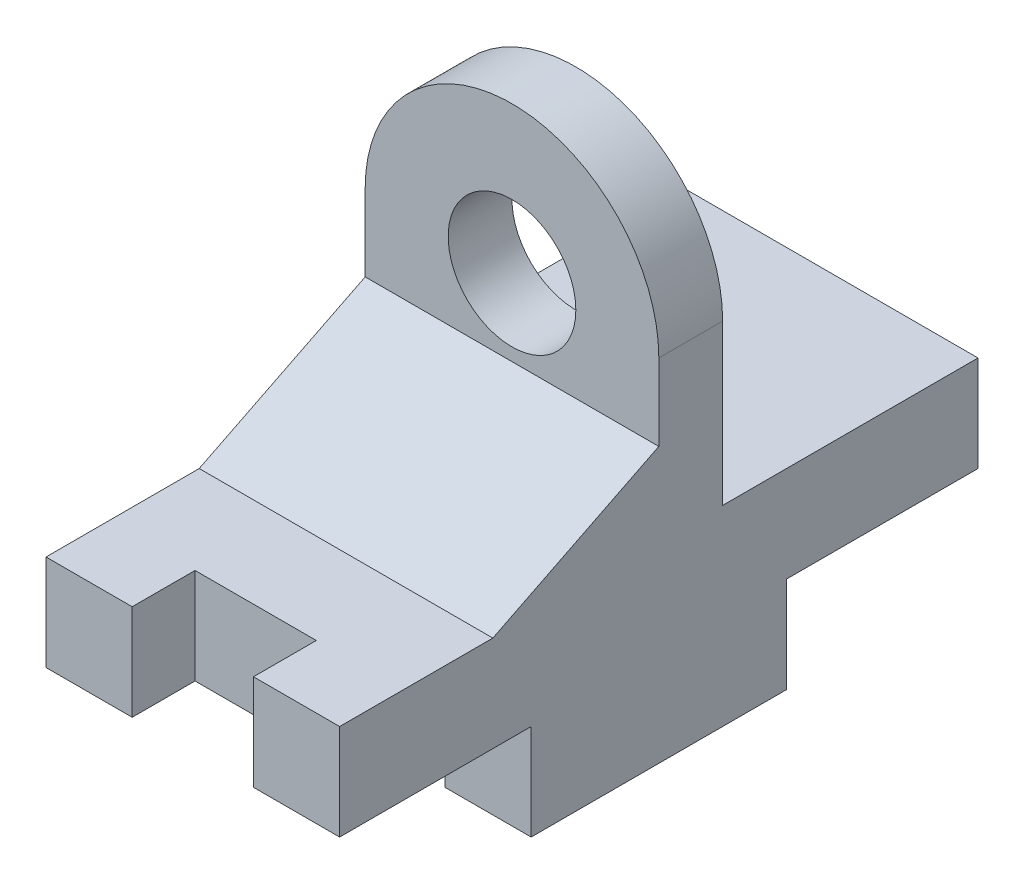
ISO-10303-21;
HEADER;
FILE_DESCRIPTION(('STEP AP214'),'2;1');
FILE_NAME('part.step','',(''),(''),'','','');
FILE_SCHEMA(('AUTOMOTIVE_DESIGN { 1 0 10303 214 1 1 1 1 }'));
ENDSEC;
DATA;
#1=APPLICATION_CONTEXT('core data for automotive mechanical design processes');
#2=APPLICATION_PROTOCOL_DEFINITION('international standard','automotive_design',2000,#1);
#3=PRODUCT_CONTEXT('',#1,'mechanical');
#4=PRODUCT('Part','Part','',(#3));
#5=PRODUCT_RELATED_PRODUCT_CATEGORY('part','',(#4));
#6=PRODUCT_DEFINITION_FORMATION('','',#4);
#7=PRODUCT_DEFINITION_CONTEXT('part definition',#1,'design');
#8=PRODUCT_DEFINITION('design','',#6,#7);
#9=PRODUCT_DEFINITION_SHAPE('','',#8);
#10=(LENGTH_UNIT() NAMED_UNIT(*) SI_UNIT(.MILLI.,.METRE.));
#11=(NAMED_UNIT(*) PLANE_ANGLE_UNIT() SI_UNIT($,.RADIAN.));
#12=(NAMED_UNIT(*) SI_UNIT($,.STERADIAN.) SOLID_ANGLE_UNIT());
#13=UNCERTAINTY_MEASURE_WITH_UNIT(LENGTH_MEASURE(1.E-05),#10,'distance_accuracy_value','');
#14=(GEOMETRIC_REPRESENTATION_CONTEXT(3) GLOBAL_UNCERTAINTY_ASSIGNED_CONTEXT((#13)) GLOBAL_UNIT_ASSIGNED_CONTEXT((#10,
#11,#12)) REPRESENTATION_CONTEXT('',''));
#15=CARTESIAN_POINT('',(0.,0.,0.));
#16=DIRECTION('',(0.,0.,1.));
#17=DIRECTION('',(1.,0.,0.));
#18=AXIS2_PLACEMENT_3D('',#15,#16,#17);
#19=CARTESIAN_POINT('',(0.,15.,0.));
#20=DIRECTION('',(0.,-1.,0.));
#21=DIRECTION('',(0.,0.,-1.));
#22=AXIS2_PLACEMENT_3D('',#19,#20,#21);
#23=PLANE('',#22);
#24=DIRECTION('',(-1.,0.,0.));
#25=VECTOR('',#24,1.);
#26=CARTESIAN_POINT('',(0.,15.,-60.));
#27=LINE('',#26,#25);
#28=CARTESIAN_POINT('',(46.,15.,-60.));
#29=VERTEX_POINT('',#28);
#30=CARTESIAN_POINT('',(0.,15.,-60.));
#31=VERTEX_POINT('',#30);
#32=EDGE_CURVE('E57',#29,#31,#27,.T.);
#33=ORIENTED_EDGE('',*,*,#32,.F.);
#34=DIRECTION('',(0.,0.,-1.));
#35=VECTOR('',#34,1.);
#36=CARTESIAN_POINT('',(46.,15.,0.));
#37=LINE('',#36,#35);
#38=CARTESIAN_POINT('',(46.,15.,-100.));
#39=VERTEX_POINT('',#38);
#40=EDGE_CURVE('E288',#29,#39,#37,.T.);
#41=ORIENTED_EDGE('',*,*,#40,.T.);
#42=DIRECTION('',(-1.,0.,0.));
#43=VECTOR('',#42,1.);
#44=CARTESIAN_POINT('',(0.,15.,-100.));
#45=LINE('',#44,#43);
#46=CARTESIAN_POINT('',(0.,15.,-100.));
#47=VERTEX_POINT('',#46);
#48=EDGE_CURVE('E291',#39,#47,#45,.T.);
#49=ORIENTED_EDGE('',*,*,#48,.T.);
#50=DIRECTION('',(0.,0.,1.));
#51=VECTOR('',#50,1.);
#52=CARTESIAN_POINT('',(0.,15.,0.));
#53=LINE('',#52,#51);
#54=EDGE_CURVE('E280',#47,#31,#53,.T.);
#55=ORIENTED_EDGE('',*,*,#54,.T.);
#56=EDGE_LOOP('',(#33,#41,#49,#55));
#57=FACE_BOUND('',#56,.T.);
#58=ADVANCED_FACE('F41',(#57),#23,.F.);
#59=CARTESIAN_POINT('',(0.,15.,0.));
#60=DIRECTION('',(1.,0.,0.));
#61=DIRECTION('',(0.,0.,-1.));
#62=AXIS2_PLACEMENT_3D('',#59,#60,#61);
#63=PLANE('',#62);
#64=CARTESIAN_POINT('',(0.,15.,-24.));
#65=VERTEX_POINT('',#64);
#66=CARTESIAN_POINT('',(0.,15.,0.));
#67=VERTEX_POINT('',#66);
#68=EDGE_CURVE('E202',#65,#67,#53,.T.);
#69=ORIENTED_EDGE('',*,*,#68,.F.);
#70=DIRECTION('',(0.,-0.447213595499958,0.894427190999916));
#71=VECTOR('',#70,1.);
#72=CARTESIAN_POINT('',(0.,15.,-24.));
#73=LINE('',#72,#71);
#74=CARTESIAN_POINT('',(0.,28.,-50.));
#75=VERTEX_POINT('',#74);
#76=EDGE_CURVE('E190',#75,#65,#73,.T.);
#77=ORIENTED_EDGE('',*,*,#76,.F.);
#78=DIRECTION('',(0.,-1.,0.));
#79=VECTOR('',#78,1.);
#80=CARTESIAN_POINT('',(0.,40.,-50.));
#81=LINE('',#80,#79);
#82=CARTESIAN_POINT('',(0.,40.,-50.));
#83=VERTEX_POINT('',#82);
#84=EDGE_CURVE('E201',#83,#75,#81,.T.);
#85=ORIENTED_EDGE('',*,*,#84,.F.);
#86=DIRECTION('',(0.,0.,1.));
#87=VECTOR('',#86,1.);
#88=CARTESIAN_POINT('',(0.,40.,0.));
#89=LINE('',#88,#87);
#90=CARTESIAN_POINT('',(0.,40.,-60.));
#91=VERTEX_POINT('',#90);
#92=EDGE_CURVE('E208',#91,#83,#89,.T.);
#93=ORIENTED_EDGE('',*,*,#92,.F.);
#94=DIRECTION('',(0.,-1.,0.));
#95=VECTOR('',#94,1.);
#96=CARTESIAN_POINT('',(0.,40.,-60.));
#97=LINE('',#96,#95);
#98=EDGE_CURVE('E209',#91,#31,#97,.T.);
#99=ORIENTED_EDGE('',*,*,#98,.T.);
#100=ORIENTED_EDGE('',*,*,#54,.F.);
#101=DIRECTION('',(0.,-1.,0.));
#102=VECTOR('',#101,1.);
#103=CARTESIAN_POINT('',(0.,15.,-100.));
#104=LINE('',#103,#102);
#105=CARTESIAN_POINT('',(0.,0.,-100.));
#106=VERTEX_POINT('',#105);
#107=EDGE_CURVE('E294',#47,#106,#104,.T.);
#108=ORIENTED_EDGE('',*,*,#107,.T.);
#109=DIRECTION('',(0.,0.,1.));
#110=VECTOR('',#109,1.);
#111=CARTESIAN_POINT('',(0.,0.,0.));
#112=LINE('',#111,#110);
#113=CARTESIAN_POINT('',(0.,0.,-70.));
#114=VERTEX_POINT('',#113);
#115=EDGE_CURVE('E298',#106,#114,#112,.T.);
#116=ORIENTED_EDGE('',*,*,#115,.T.);
#117=DIRECTION('',(0.,1.,0.));
#118=VECTOR('',#117,1.);
#119=CARTESIAN_POINT('',(0.,0.,-70.));
#120=LINE('',#119,#118);
#121=CARTESIAN_POINT('',(0.,-15.,-70.));
#122=VERTEX_POINT('',#121);
#123=EDGE_CURVE('E251',#122,#114,#120,.T.);
#124=ORIENTED_EDGE('',*,*,#123,.F.);
#125=DIRECTION('',(0.,0.,-1.));
#126=VECTOR('',#125,1.);
#127=CARTESIAN_POINT('',(0.,-15.,-70.));
#128=LINE('',#127,#126);
#129=CARTESIAN_POINT('',(0.,-15.,-30.));
#130=VERTEX_POINT('',#129);
#131=EDGE_CURVE('E264',#130,#122,#128,.T.);
#132=ORIENTED_EDGE('',*,*,#131,.F.);
#133=DIRECTION('',(0.,-1.,0.));
#134=VECTOR('',#133,1.);
#135=CARTESIAN_POINT('',(0.,-15.,-30.));
#136=LINE('',#135,#134);
#137=CARTESIAN_POINT('',(0.,0.,-30.));
#138=VERTEX_POINT('',#137);
#139=EDGE_CURVE('E242',#138,#130,#136,.T.);
#140=ORIENTED_EDGE('',*,*,#139,.F.);
#141=CARTESIAN_POINT('',(0.,0.,0.));
#142=VERTEX_POINT('',#141);
#143=EDGE_CURVE('E277',#138,#142,#112,.T.);
#144=ORIENTED_EDGE('',*,*,#143,.T.);
#145=DIRECTION('',(0.,-1.,0.));
#146=VECTOR('',#145,1.);
#147=CARTESIAN_POINT('',(0.,15.,0.));
#148=LINE('',#147,#146);
#149=EDGE_CURVE('E11',#67,#142,#148,.T.);
#150=ORIENTED_EDGE('',*,*,#149,.F.);
#151=EDGE_LOOP('',(#69,#77,#85,#93,#99,#100,#108,#116,#124,#132,#140,#144,#150));
#152=FACE_BOUND('',#151,.T.);
#153=ADVANCED_FACE('F43',(#152),#63,.F.);
#154=CARTESIAN_POINT('',(0.,15.,0.));
#155=DIRECTION('',(0.,0.,-1.));
#156=DIRECTION('',(-1.,0.,0.));
#157=AXIS2_PLACEMENT_3D('',#154,#155,#156);
#158=PLANE('',#157);
#159=DIRECTION('',(1.,0.,0.));
#160=VECTOR('',#159,1.);
#161=CARTESIAN_POINT('',(0.,0.,0.));
#162=LINE('',#161,#160);
#163=CARTESIAN_POINT('',(13.5,0.,0.));
#164=VERTEX_POINT('',#163);
#165=EDGE_CURVE('E299',#142,#164,#162,.T.);
#166=ORIENTED_EDGE('',*,*,#165,.T.);
#167=DIRECTION('',(0.,-1.,0.));
#168=VECTOR('',#167,1.);
#169=CARTESIAN_POINT('',(13.5,15.,0.));
#170=LINE('',#169,#168);
#171=CARTESIAN_POINT('',(13.5,15.,0.));
#172=VERTEX_POINT('',#171);
#173=EDGE_CURVE('E47',#172,#164,#170,.T.);
#174=ORIENTED_EDGE('',*,*,#173,.F.);
#175=DIRECTION('',(1.,0.,0.));
#176=VECTOR('',#175,1.);
#177=CARTESIAN_POINT('',(0.,15.,0.));
#178=LINE('',#177,#176);
#179=EDGE_CURVE('E276',#67,#172,#178,.T.);
#180=ORIENTED_EDGE('',*,*,#179,.F.);
#181=ORIENTED_EDGE('',*,*,#149,.T.);
#182=EDGE_LOOP('',(#166,#174,#180,#181));
#183=FACE_BOUND('',#182,.T.);
#184=ADVANCED_FACE('F360',(#183),#158,.F.);
#185=CARTESIAN_POINT('',(13.5,15.,0.));
#186=DIRECTION('',(-1.,0.,0.));
#187=DIRECTION('',(0.,0.,1.));
#188=AXIS2_PLACEMENT_3D('',#185,#186,#187);
#189=PLANE('',#188);
#190=DIRECTION('',(0.,0.,-1.));
#191=VECTOR('',#190,1.);
#192=CARTESIAN_POINT('',(13.5,0.,0.));
#193=LINE('',#192,#191);
#194=CARTESIAN_POINT('',(13.5,0.,-9.84759162992863));
#195=VERTEX_POINT('',#194);
#196=EDGE_CURVE('E301',#164,#195,#193,.T.);
#197=ORIENTED_EDGE('',*,*,#196,.T.);
#198=DIRECTION('',(0.,-1.,0.));
#199=VECTOR('',#198,1.);
#200=CARTESIAN_POINT('',(13.5,15.,-9.84759162992863));
#201=LINE('',#200,#199);
#202=CARTESIAN_POINT('',(13.5,15.,-9.84759162992863));
#203=VERTEX_POINT('',#202);
#204=EDGE_CURVE('E326',#203,#195,#201,.T.);
#205=ORIENTED_EDGE('',*,*,#204,.F.);
#206=DIRECTION('',(0.,0.,-1.));
#207=VECTOR('',#206,1.);
#208=CARTESIAN_POINT('',(13.5,15.,0.));
#209=LINE('',#208,#207);
#210=EDGE_CURVE('E282',#172,#203,#209,.T.);
#211=ORIENTED_EDGE('',*,*,#210,.F.);
#212=ORIENTED_EDGE('',*,*,#173,.T.);
#213=EDGE_LOOP('',(#197,#205,#211,#212));
#214=FACE_BOUND('',#213,.T.);
#215=ADVANCED_FACE('F337',(#214),#189,.F.);
#216=CARTESIAN_POINT('',(13.5,15.,-9.84759162992863));
#217=DIRECTION('',(0.,0.,-1.));
#218=DIRECTION('',(-1.,0.,0.));
#219=AXIS2_PLACEMENT_3D('',#216,#217,#218);
#220=PLANE('',#219);
#221=DIRECTION('',(1.,0.,0.));
#222=VECTOR('',#221,1.);
#223=CARTESIAN_POINT('',(13.5,0.,-9.84759162992863));
#224=LINE('',#223,#222);
#225=CARTESIAN_POINT('',(32.5,0.,-9.84759162992863));
#226=VERTEX_POINT('',#225);
#227=EDGE_CURVE('E303',#195,#226,#224,.T.);
#228=ORIENTED_EDGE('',*,*,#227,.T.);
#229=DIRECTION('',(0.,-1.,0.));
#230=VECTOR('',#229,1.);
#231=CARTESIAN_POINT('',(32.5,15.,-9.84759162992863));
#232=LINE('',#231,#230);
#233=CARTESIAN_POINT('',(32.5,15.,-9.84759162992863));
#234=VERTEX_POINT('',#233);
#235=EDGE_CURVE('E327',#234,#226,#232,.T.);
#236=ORIENTED_EDGE('',*,*,#235,.F.);
#237=DIRECTION('',(1.,0.,0.));
#238=VECTOR('',#237,1.);
#239=CARTESIAN_POINT('',(13.5,15.,-9.84759162992863));
#240=LINE('',#239,#238);
#241=EDGE_CURVE('E284',#203,#234,#240,.T.);
#242=ORIENTED_EDGE('',*,*,#241,.F.);
#243=ORIENTED_EDGE('',*,*,#204,.T.);
#244=EDGE_LOOP('',(#228,#236,#242,#243));
#245=FACE_BOUND('',#244,.T.);
#246=ADVANCED_FACE('F346',(#245),#220,.F.);
#247=CARTESIAN_POINT('',(32.5,15.,-9.84759162992863));
#248=DIRECTION('',(1.,0.,0.));
#249=DIRECTION('',(0.,0.,-1.));
#250=AXIS2_PLACEMENT_3D('',#247,#248,#249);
#251=PLANE('',#250);
#252=DIRECTION('',(0.,0.,1.));
#253=VECTOR('',#252,1.);
#254=CARTESIAN_POINT('',(32.5,0.,-9.84759162992863));
#255=LINE('',#254,#253);
#256=CARTESIAN_POINT('',(32.5,0.,0.));
#257=VERTEX_POINT('',#256);
#258=EDGE_CURVE('E304',#226,#257,#255,.T.);
#259=ORIENTED_EDGE('',*,*,#258,.T.);
#260=DIRECTION('',(0.,-1.,0.));
#261=VECTOR('',#260,1.);
#262=CARTESIAN_POINT('',(32.5,15.,0.));
#263=LINE('',#262,#261);
#264=CARTESIAN_POINT('',(32.5,15.,0.));
#265=VERTEX_POINT('',#264);
#266=EDGE_CURVE('E324',#265,#257,#263,.T.);
#267=ORIENTED_EDGE('',*,*,#266,.F.);
#268=DIRECTION('',(0.,0.,1.));
#269=VECTOR('',#268,1.);
#270=CARTESIAN_POINT('',(32.5,15.,-9.84759162992863));
#271=LINE('',#270,#269);
#272=EDGE_CURVE('E283',#234,#265,#271,.T.);
#273=ORIENTED_EDGE('',*,*,#272,.F.);
#274=ORIENTED_EDGE('',*,*,#235,.T.);
#275=EDGE_LOOP('',(#259,#267,#273,#274));
#276=FACE_BOUND('',#275,.T.);
#277=ADVANCED_FACE('F352',(#276),#251,.F.);
#278=CARTESIAN_POINT('',(32.5,15.,0.));
#279=DIRECTION('',(0.,0.,-1.));
#280=DIRECTION('',(-1.,0.,0.));
#281=AXIS2_PLACEMENT_3D('',#278,#279,#280);
#282=PLANE('',#281);
#283=DIRECTION('',(1.,0.,0.));
#284=VECTOR('',#283,1.);
#285=CARTESIAN_POINT('',(32.5,0.,0.));
#286=LINE('',#285,#284);
#287=CARTESIAN_POINT('',(46.,0.,0.));
#288=VERTEX_POINT('',#287);
#289=EDGE_CURVE('E310',#257,#288,#286,.T.);
#290=ORIENTED_EDGE('',*,*,#289,.T.);
#291=DIRECTION('',(0.,-1.,0.));
#292=VECTOR('',#291,1.);
#293=CARTESIAN_POINT('',(46.,15.,0.));
#294=LINE('',#293,#292);
#295=CARTESIAN_POINT('',(46.,15.,0.));
#296=VERTEX_POINT('',#295);
#297=EDGE_CURVE('E318',#296,#288,#294,.T.);
#298=ORIENTED_EDGE('',*,*,#297,.F.);
#299=DIRECTION('',(1.,0.,0.));
#300=VECTOR('',#299,1.);
#301=CARTESIAN_POINT('',(32.5,15.,0.));
#302=LINE('',#301,#300);
#303=EDGE_CURVE('E290',#265,#296,#302,.T.);
#304=ORIENTED_EDGE('',*,*,#303,.F.);
#305=ORIENTED_EDGE('',*,*,#266,.T.);
#306=EDGE_LOOP('',(#290,#298,#304,#305));
#307=FACE_BOUND('',#306,.T.);
#308=ADVANCED_FACE('F454',(#307),#282,.F.);
#309=CARTESIAN_POINT('',(46.,15.,0.));
#310=DIRECTION('',(-1.,0.,0.));
#311=DIRECTION('',(0.,0.,1.));
#312=AXIS2_PLACEMENT_3D('',#309,#310,#311);
#313=PLANE('',#312);
#314=DIRECTION('',(0.,0.,-1.));
#315=VECTOR('',#314,1.);
#316=CARTESIAN_POINT('',(46.,0.,0.));
#317=LINE('',#316,#315);
#318=CARTESIAN_POINT('',(46.,0.,-30.));
#319=VERTEX_POINT('',#318);
#320=EDGE_CURVE('E309',#288,#319,#317,.T.);
#321=ORIENTED_EDGE('',*,*,#320,.T.);
#322=DIRECTION('',(0.,-1.,0.));
#323=VECTOR('',#322,1.);
#324=CARTESIAN_POINT('',(46.,-15.,-30.));
#325=LINE('',#324,#323);
#326=CARTESIAN_POINT('',(46.,-15.,-30.));
#327=VERTEX_POINT('',#326);
#328=EDGE_CURVE('E222',#319,#327,#325,.T.);
#329=ORIENTED_EDGE('',*,*,#328,.T.);
#330=DIRECTION('',(0.,0.,-1.));
#331=VECTOR('',#330,1.);
#332=CARTESIAN_POINT('',(46.,-15.,-70.));
#333=LINE('',#332,#331);
#334=CARTESIAN_POINT('',(46.,-15.,-70.));
#335=VERTEX_POINT('',#334);
#336=EDGE_CURVE('E238',#327,#335,#333,.T.);
#337=ORIENTED_EDGE('',*,*,#336,.T.);
#338=DIRECTION('',(0.,1.,0.));
#339=VECTOR('',#338,1.);
#340=CARTESIAN_POINT('',(46.,0.,-70.));
#341=LINE('',#340,#339);
#342=CARTESIAN_POINT('',(46.,0.,-70.));
#343=VERTEX_POINT('',#342);
#344=EDGE_CURVE('E61',#335,#343,#341,.T.);
#345=ORIENTED_EDGE('',*,*,#344,.T.);
#346=CARTESIAN_POINT('',(46.,0.,-100.));
#347=VERTEX_POINT('',#346);
#348=EDGE_CURVE('E307',#343,#347,#317,.T.);
#349=ORIENTED_EDGE('',*,*,#348,.T.);
#350=DIRECTION('',(0.,-1.,0.));
#351=VECTOR('',#350,1.);
#352=CARTESIAN_POINT('',(46.,15.,-100.));
#353=LINE('',#352,#351);
#354=EDGE_CURVE('E320',#39,#347,#353,.T.);
#355=ORIENTED_EDGE('',*,*,#354,.F.);
#356=ORIENTED_EDGE('',*,*,#40,.F.);
#357=DIRECTION('',(0.,-1.,0.));
#358=VECTOR('',#357,1.);
#359=CARTESIAN_POINT('',(46.,40.,-60.));
#360=LINE('',#359,#358);
#361=CARTESIAN_POINT('',(46.,40.,-60.));
#362=VERTEX_POINT('',#361);
#363=EDGE_CURVE('E214',#362,#29,#360,.T.);
#364=ORIENTED_EDGE('',*,*,#363,.F.);
#365=DIRECTION('',(0.,0.,-1.));
#366=VECTOR('',#365,1.);
#367=CARTESIAN_POINT('',(46.,40.,0.));
#368=LINE('',#367,#366);
#369=CARTESIAN_POINT('',(46.,40.,-50.));
#370=VERTEX_POINT('',#369);
#371=EDGE_CURVE('E213',#370,#362,#368,.T.);
#372=ORIENTED_EDGE('',*,*,#371,.F.);
#373=DIRECTION('',(0.,-1.,0.));
#374=VECTOR('',#373,1.);
#375=CARTESIAN_POINT('',(46.,40.,-50.));
#376=LINE('',#375,#374);
#377=CARTESIAN_POINT('',(46.,28.,-50.));
#378=VERTEX_POINT('',#377);
#379=EDGE_CURVE('E221',#370,#378,#376,.T.);
#380=ORIENTED_EDGE('',*,*,#379,.T.);
#381=DIRECTION('',(0.,-0.447213595499958,0.894427190999916));
#382=VECTOR('',#381,1.);
#383=CARTESIAN_POINT('',(46.,15.,-24.));
#384=LINE('',#383,#382);
#385=CARTESIAN_POINT('',(46.,15.,-24.));
#386=VERTEX_POINT('',#385);
#387=EDGE_CURVE('E188',#378,#386,#384,.T.);
#388=ORIENTED_EDGE('',*,*,#387,.T.);
#389=EDGE_CURVE('E289',#296,#386,#37,.T.);
#390=ORIENTED_EDGE('',*,*,#389,.F.);
#391=ORIENTED_EDGE('',*,*,#297,.T.);
#392=EDGE_LOOP('',(#321,#329,#337,#345,#349,#355,#356,#364,#372,#380,#388,#390,#391));
#393=FACE_BOUND('',#392,.T.);
#394=ADVANCED_FACE('F383',(#393),#313,.F.);
#395=CARTESIAN_POINT('',(0.,15.,-100.));
#396=DIRECTION('',(0.,0.,1.));
#397=DIRECTION('',(1.,0.,0.));
#398=AXIS2_PLACEMENT_3D('',#395,#396,#397);
#399=PLANE('',#398);
#400=DIRECTION('',(-1.,0.,0.));
#401=VECTOR('',#400,1.);
#402=CARTESIAN_POINT('',(0.,0.,-100.));
#403=LINE('',#402,#401);
#404=EDGE_CURVE('E312',#347,#106,#403,.T.);
#405=ORIENTED_EDGE('',*,*,#404,.T.);
#406=ORIENTED_EDGE('',*,*,#107,.F.);
#407=ORIENTED_EDGE('',*,*,#48,.F.);
#408=ORIENTED_EDGE('',*,*,#354,.T.);
#409=EDGE_LOOP('',(#405,#406,#407,#408));
#410=FACE_BOUND('',#409,.T.);
#411=ADVANCED_FACE('F382',(#410),#399,.F.);
#412=ORIENTED_EDGE('',*,*,#389,.T.);
#413=DIRECTION('',(1.,0.,0.));
#414=VECTOR('',#413,1.);
#415=CARTESIAN_POINT('',(0.,15.,-24.));
#416=LINE('',#415,#414);
#417=EDGE_CURVE('E193',#65,#386,#416,.T.);
#418=ORIENTED_EDGE('',*,*,#417,.F.);
#419=ORIENTED_EDGE('',*,*,#68,.T.);
#420=ORIENTED_EDGE('',*,*,#179,.T.);
#421=ORIENTED_EDGE('',*,*,#210,.T.);
#422=ORIENTED_EDGE('',*,*,#241,.T.);
#423=ORIENTED_EDGE('',*,*,#272,.T.);
#424=ORIENTED_EDGE('',*,*,#303,.T.);
#425=EDGE_LOOP('',(#412,#418,#419,#420,#421,#422,#423,#424));
#426=FACE_BOUND('',#425,.T.);
#427=ADVANCED_FACE('F357',(#426),#23,.F.);
#428=CARTESIAN_POINT('',(0.,0.,0.));
#429=DIRECTION('',(0.,-1.,0.));
#430=DIRECTION('',(0.,0.,-1.));
#431=AXIS2_PLACEMENT_3D('',#428,#429,#430);
#432=PLANE('',#431);
#433=DIRECTION('',(1.,0.,0.));
#434=VECTOR('',#433,1.);
#435=CARTESIAN_POINT('',(32.5,0.,-30.));
#436=LINE('',#435,#434);
#437=CARTESIAN_POINT('',(32.5,0.,-30.));
#438=VERTEX_POINT('',#437);
#439=EDGE_CURVE('E241',#438,#319,#436,.T.);
#440=ORIENTED_EDGE('',*,*,#439,.T.);
#441=ORIENTED_EDGE('',*,*,#320,.F.);
#442=ORIENTED_EDGE('',*,*,#289,.F.);
#443=ORIENTED_EDGE('',*,*,#258,.F.);
#444=ORIENTED_EDGE('',*,*,#227,.F.);
#445=ORIENTED_EDGE('',*,*,#196,.F.);
#446=ORIENTED_EDGE('',*,*,#165,.F.);
#447=ORIENTED_EDGE('',*,*,#143,.F.);
#448=DIRECTION('',(-1.,0.,0.));
#449=VECTOR('',#448,1.);
#450=CARTESIAN_POINT('',(13.5,0.,-30.));
#451=LINE('',#450,#449);
#452=CARTESIAN_POINT('',(13.5,0.,-30.));
#453=VERTEX_POINT('',#452);
#454=EDGE_CURVE('E258',#453,#138,#451,.T.);
#455=ORIENTED_EDGE('',*,*,#454,.F.);
#456=DIRECTION('',(0.,0.,1.));
#457=VECTOR('',#456,1.);
#458=CARTESIAN_POINT('',(13.5,0.,-30.));
#459=LINE('',#458,#457);
#460=CARTESIAN_POINT('',(13.5,0.,-70.));
#461=VERTEX_POINT('',#460);
#462=EDGE_CURVE('E259',#461,#453,#459,.T.);
#463=ORIENTED_EDGE('',*,*,#462,.F.);
#464=DIRECTION('',(-1.,0.,0.));
#465=VECTOR('',#464,1.);
#466=CARTESIAN_POINT('',(13.5,0.,-70.));
#467=LINE('',#466,#465);
#468=EDGE_CURVE('E270',#461,#114,#467,.T.);
#469=ORIENTED_EDGE('',*,*,#468,.T.);
#470=ORIENTED_EDGE('',*,*,#115,.F.);
#471=ORIENTED_EDGE('',*,*,#404,.F.);
#472=ORIENTED_EDGE('',*,*,#348,.F.);
#473=DIRECTION('',(1.,0.,0.));
#474=VECTOR('',#473,1.);
#475=CARTESIAN_POINT('',(32.5,0.,-70.));
#476=LINE('',#475,#474);
#477=CARTESIAN_POINT('',(32.5,0.,-70.));
#478=VERTEX_POINT('',#477);
#479=EDGE_CURVE('E244',#478,#343,#476,.T.);
#480=ORIENTED_EDGE('',*,*,#479,.F.);
#481=DIRECTION('',(0.,0.,1.));
#482=VECTOR('',#481,1.);
#483=CARTESIAN_POINT('',(32.5,0.,-30.));
#484=LINE('',#483,#482);
#485=EDGE_CURVE('E235',#478,#438,#484,.T.);
#486=ORIENTED_EDGE('',*,*,#485,.T.);
#487=EDGE_LOOP('',(#440,#441,#442,#443,#444,#445,#446,#447,#455,#463,#469,#470,#471,#472,#480,#486));
#488=FACE_BOUND('',#487,.T.);
#489=ADVANCED_FACE('F344',(#488),#432,.T.);
#490=CARTESIAN_POINT('',(13.5,-15.,-30.));
#491=DIRECTION('',(0.,0.,-1.));
#492=DIRECTION('',(0.,1.,0.));
#493=AXIS2_PLACEMENT_3D('',#490,#491,#492);
#494=PLANE('',#493);
#495=ORIENTED_EDGE('',*,*,#139,.T.);
#496=DIRECTION('',(-1.,0.,0.));
#497=VECTOR('',#496,1.);
#498=CARTESIAN_POINT('',(13.5,-15.,-30.));
#499=LINE('',#498,#497);
#500=CARTESIAN_POINT('',(13.5,-15.,-30.));
#501=VERTEX_POINT('',#500);
#502=EDGE_CURVE('E271',#501,#130,#499,.T.);
#503=ORIENTED_EDGE('',*,*,#502,.F.);
#504=DIRECTION('',(0.,-1.,0.));
#505=VECTOR('',#504,1.);
#506=CARTESIAN_POINT('',(13.5,-15.,-30.));
#507=LINE('',#506,#505);
#508=EDGE_CURVE('E249',#453,#501,#507,.T.);
#509=ORIENTED_EDGE('',*,*,#508,.F.);
#510=ORIENTED_EDGE('',*,*,#454,.T.);
#511=EDGE_LOOP('',(#495,#503,#509,#510));
#512=FACE_BOUND('',#511,.T.);
#513=ADVANCED_FACE('F362',(#512),#494,.F.);
#514=CARTESIAN_POINT('',(13.5,-15.,-70.));
#515=DIRECTION('',(0.,1.,0.));
#516=DIRECTION('',(0.,0.,1.));
#517=AXIS2_PLACEMENT_3D('',#514,#515,#516);
#518=PLANE('',#517);
#519=ORIENTED_EDGE('',*,*,#131,.T.);
#520=DIRECTION('',(-1.,0.,0.));
#521=VECTOR('',#520,1.);
#522=CARTESIAN_POINT('',(13.5,-15.,-70.));
#523=LINE('',#522,#521);
#524=CARTESIAN_POINT('',(13.5,-15.,-70.));
#525=VERTEX_POINT('',#524);
#526=EDGE_CURVE('E269',#525,#122,#523,.T.);
#527=ORIENTED_EDGE('',*,*,#526,.F.);
#528=DIRECTION('',(0.,0.,-1.));
#529=VECTOR('',#528,1.);
#530=CARTESIAN_POINT('',(13.5,-15.,-70.));
#531=LINE('',#530,#529);
#532=EDGE_CURVE('E254',#501,#525,#531,.T.);
#533=ORIENTED_EDGE('',*,*,#532,.F.);
#534=ORIENTED_EDGE('',*,*,#502,.T.);
#535=EDGE_LOOP('',(#519,#527,#533,#534));
#536=FACE_BOUND('',#535,.T.);
#537=ADVANCED_FACE('F535',(#536),#518,.F.);
#538=CARTESIAN_POINT('',(13.5,0.,-70.));
#539=DIRECTION('',(0.,0.,1.));
#540=DIRECTION('',(1.,0.,0.));
#541=AXIS2_PLACEMENT_3D('',#538,#539,#540);
#542=PLANE('',#541);
#543=ORIENTED_EDGE('',*,*,#123,.T.);
#544=ORIENTED_EDGE('',*,*,#468,.F.);
#545=DIRECTION('',(0.,1.,0.));
#546=VECTOR('',#545,1.);
#547=CARTESIAN_POINT('',(13.5,0.,-70.));
#548=LINE('',#547,#546);
#549=EDGE_CURVE('E257',#525,#461,#548,.T.);
#550=ORIENTED_EDGE('',*,*,#549,.F.);
#551=ORIENTED_EDGE('',*,*,#526,.T.);
#552=EDGE_LOOP('',(#543,#544,#550,#551));
#553=FACE_BOUND('',#552,.T.);
#554=ADVANCED_FACE('F373',(#553),#542,.F.);
#555=CARTESIAN_POINT('',(13.5,0.,0.));
#556=DIRECTION('',(-1.,0.,0.));
#557=DIRECTION('',(0.,0.,1.));
#558=AXIS2_PLACEMENT_3D('',#555,#556,#557);
#559=PLANE('',#558);
#560=ORIENTED_EDGE('',*,*,#508,.T.);
#561=ORIENTED_EDGE('',*,*,#532,.T.);
#562=ORIENTED_EDGE('',*,*,#549,.T.);
#563=ORIENTED_EDGE('',*,*,#462,.T.);
#564=EDGE_LOOP('',(#560,#561,#562,#563));
#565=FACE_BOUND('',#564,.T.);
#566=ADVANCED_FACE('F368',(#565),#559,.F.);
#567=CARTESIAN_POINT('',(32.5,-15.,-30.));
#568=DIRECTION('',(0.,0.,1.));
#569=DIRECTION('',(0.,-1.,0.));
#570=AXIS2_PLACEMENT_3D('',#567,#568,#569);
#571=PLANE('',#570);
#572=ORIENTED_EDGE('',*,*,#328,.F.);
#573=ORIENTED_EDGE('',*,*,#439,.F.);
#574=DIRECTION('',(0.,-1.,0.));
#575=VECTOR('',#574,1.);
#576=CARTESIAN_POINT('',(32.5,-15.,-30.));
#577=LINE('',#576,#575);
#578=CARTESIAN_POINT('',(32.5,-15.,-30.));
#579=VERTEX_POINT('',#578);
#580=EDGE_CURVE('E223',#438,#579,#577,.T.);
#581=ORIENTED_EDGE('',*,*,#580,.T.);
#582=DIRECTION('',(1.,0.,0.));
#583=VECTOR('',#582,1.);
#584=CARTESIAN_POINT('',(32.5,-15.,-30.));
#585=LINE('',#584,#583);
#586=EDGE_CURVE('E232',#579,#327,#585,.T.);
#587=ORIENTED_EDGE('',*,*,#586,.T.);
#588=EDGE_LOOP('',(#572,#573,#581,#587));
#589=FACE_BOUND('',#588,.T.);
#590=ADVANCED_FACE('F414',(#589),#571,.T.);
#591=CARTESIAN_POINT('',(32.5,0.,-70.));
#592=DIRECTION('',(0.,0.,-1.));
#593=DIRECTION('',(-1.,0.,0.));
#594=AXIS2_PLACEMENT_3D('',#591,#592,#593);
#595=PLANE('',#594);
#596=ORIENTED_EDGE('',*,*,#344,.F.);
#597=DIRECTION('',(1.,0.,0.));
#598=VECTOR('',#597,1.);
#599=CARTESIAN_POINT('',(32.5,-15.,-70.));
#600=LINE('',#599,#598);
#601=CARTESIAN_POINT('',(32.5,-15.,-70.));
#602=VERTEX_POINT('',#601);
#603=EDGE_CURVE('E250',#602,#335,#600,.T.);
#604=ORIENTED_EDGE('',*,*,#603,.F.);
#605=DIRECTION('',(0.,1.,0.));
#606=VECTOR('',#605,1.);
#607=CARTESIAN_POINT('',(32.5,0.,-70.));
#608=LINE('',#607,#606);
#609=EDGE_CURVE('E229',#602,#478,#608,.T.);
#610=ORIENTED_EDGE('',*,*,#609,.T.);
#611=ORIENTED_EDGE('',*,*,#479,.T.);
#612=EDGE_LOOP('',(#596,#604,#610,#611));
#613=FACE_BOUND('',#612,.T.);
#614=ADVANCED_FACE('F422',(#613),#595,.T.);
#615=CARTESIAN_POINT('',(32.5,-15.,-70.));
#616=DIRECTION('',(0.,-1.,0.));
#617=DIRECTION('',(0.,0.,-1.));
#618=AXIS2_PLACEMENT_3D('',#615,#616,#617);
#619=PLANE('',#618);
#620=ORIENTED_EDGE('',*,*,#336,.F.);
#621=ORIENTED_EDGE('',*,*,#586,.F.);
#622=DIRECTION('',(0.,0.,-1.));
#623=VECTOR('',#622,1.);
#624=CARTESIAN_POINT('',(32.5,-15.,-70.));
#625=LINE('',#624,#623);
#626=EDGE_CURVE('E227',#579,#602,#625,.T.);
#627=ORIENTED_EDGE('',*,*,#626,.T.);
#628=ORIENTED_EDGE('',*,*,#603,.T.);
#629=EDGE_LOOP('',(#620,#621,#627,#628));
#630=FACE_BOUND('',#629,.T.);
#631=ADVANCED_FACE('F419',(#630),#619,.T.);
#632=CARTESIAN_POINT('',(32.5,0.,0.));
#633=DIRECTION('',(-1.,0.,0.));
#634=DIRECTION('',(0.,0.,1.));
#635=AXIS2_PLACEMENT_3D('',#632,#633,#634);
#636=PLANE('',#635);
#637=ORIENTED_EDGE('',*,*,#580,.F.);
#638=ORIENTED_EDGE('',*,*,#485,.F.);
#639=ORIENTED_EDGE('',*,*,#609,.F.);
#640=ORIENTED_EDGE('',*,*,#626,.F.);
#641=EDGE_LOOP('',(#637,#638,#639,#640));
#642=FACE_BOUND('',#641,.T.);
#643=ADVANCED_FACE('F416',(#642),#636,.T.);
#644=CARTESIAN_POINT('',(0.,40.,-50.));
#645=DIRECTION('',(0.,0.,1.));
#646=DIRECTION('',(1.,0.,0.));
#647=AXIS2_PLACEMENT_3D('',#644,#645,#646);
#648=PLANE('',#647);
#649=DIRECTION('',(1.,0.,0.));
#650=VECTOR('',#649,1.);
#651=CARTESIAN_POINT('',(0.,28.,-50.));
#652=LINE('',#651,#650);
#653=EDGE_CURVE('E183',#75,#378,#652,.T.);
#654=ORIENTED_EDGE('',*,*,#653,.T.);
#655=ORIENTED_EDGE('',*,*,#379,.F.);
#656=CARTESIAN_POINT('',(23.,40.,-50.));
#657=DIRECTION('',(0.,0.,1.));
#658=DIRECTION('',(1.,0.,0.));
#659=AXIS2_PLACEMENT_3D('',#656,#657,#658);
#660=CIRCLE('',#659,23.);
#661=EDGE_CURVE('E210',#370,#83,#660,.T.);
#662=ORIENTED_EDGE('',*,*,#661,.T.);
#663=ORIENTED_EDGE('',*,*,#84,.T.);
#664=EDGE_LOOP('',(#654,#655,#662,#663));
#665=FACE_BOUND('',#664,.T.);
#666=CARTESIAN_POINT('',(23.,40.,-50.));
#667=DIRECTION('',(0.,0.,1.));
#668=DIRECTION('',(1.,0.,0.));
#669=AXIS2_PLACEMENT_3D('',#666,#667,#668);
#670=CIRCLE('',#669,10.);
#671=CARTESIAN_POINT('',(33.,40.,-50.));
#672=VERTEX_POINT('',#671);
#673=EDGE_CURVE('E399',#672,#672,#670,.T.);
#674=ORIENTED_EDGE('',*,*,#673,.F.);
#675=EDGE_LOOP('',(#674));
#676=FACE_BOUND('',#675,.T.);
#677=ADVANCED_FACE('F204',(#665,#676),#648,.T.);
#678=CARTESIAN_POINT('',(0.,40.,-60.));
#679=DIRECTION('',(0.,0.,1.));
#680=DIRECTION('',(1.,0.,0.));
#681=AXIS2_PLACEMENT_3D('',#678,#679,#680);
#682=PLANE('',#681);
#683=ORIENTED_EDGE('',*,*,#98,.F.);
#684=CARTESIAN_POINT('',(23.,40.,-60.));
#685=DIRECTION('',(0.,0.,1.));
#686=DIRECTION('',(1.,0.,0.));
#687=AXIS2_PLACEMENT_3D('',#684,#685,#686);
#688=CIRCLE('',#687,23.);
#689=EDGE_CURVE('E394',#362,#91,#688,.T.);
#690=ORIENTED_EDGE('',*,*,#689,.F.);
#691=ORIENTED_EDGE('',*,*,#363,.T.);
#692=ORIENTED_EDGE('',*,*,#32,.T.);
#693=EDGE_LOOP('',(#683,#690,#691,#692));
#694=FACE_BOUND('',#693,.T.);
#695=CARTESIAN_POINT('',(23.,40.,-60.));
#696=DIRECTION('',(0.,0.,1.));
#697=DIRECTION('',(1.,0.,0.));
#698=AXIS2_PLACEMENT_3D('',#695,#696,#697);
#699=CIRCLE('',#698,10.);
#700=CARTESIAN_POINT('',(33.,40.,-60.));
#701=VERTEX_POINT('',#700);
#702=EDGE_CURVE('E393',#701,#701,#699,.T.);
#703=ORIENTED_EDGE('',*,*,#702,.T.);
#704=EDGE_LOOP('',(#703));
#705=FACE_BOUND('',#704,.T.);
#706=ADVANCED_FACE('F392',(#694,#705),#682,.F.);
#707=CARTESIAN_POINT('',(23.,40.,-60.));
#708=DIRECTION('',(0.,0.,1.));
#709=DIRECTION('',(1.,0.,0.));
#710=AXIS2_PLACEMENT_3D('',#707,#708,#709);
#711=CYLINDRICAL_SURFACE('',#710,10.);
#712=ORIENTED_EDGE('',*,*,#673,.T.);
#713=EDGE_LOOP('',(#712));
#714=FACE_BOUND('',#713,.T.);
#715=ORIENTED_EDGE('',*,*,#702,.F.);
#716=EDGE_LOOP('',(#715));
#717=FACE_BOUND('',#716,.T.);
#718=ADVANCED_FACE('F591',(#714,#717),#711,.F.);
#719=CARTESIAN_POINT('',(23.,40.,-60.));
#720=DIRECTION('',(0.,0.,1.));
#721=DIRECTION('',(1.,0.,0.));
#722=AXIS2_PLACEMENT_3D('',#719,#720,#721);
#723=CYLINDRICAL_SURFACE('',#722,23.);
#724=ORIENTED_EDGE('',*,*,#661,.F.);
#725=ORIENTED_EDGE('',*,*,#371,.T.);
#726=ORIENTED_EDGE('',*,*,#689,.T.);
#727=ORIENTED_EDGE('',*,*,#92,.T.);
#728=EDGE_LOOP('',(#724,#725,#726,#727));
#729=FACE_BOUND('',#728,.T.);
#730=ADVANCED_FACE('F404',(#729),#723,.T.);
#731=CARTESIAN_POINT('',(0.,15.,-24.));
#732=DIRECTION('',(0.,0.894427190999916,0.447213595499958));
#733=DIRECTION('',(0.,-0.447213595499958,0.894427190999916));
#734=AXIS2_PLACEMENT_3D('',#731,#732,#733);
#735=PLANE('',#734);
#736=ORIENTED_EDGE('',*,*,#387,.F.);
#737=ORIENTED_EDGE('',*,*,#653,.F.);
#738=ORIENTED_EDGE('',*,*,#76,.T.);
#739=ORIENTED_EDGE('',*,*,#417,.T.);
#740=EDGE_LOOP('',(#736,#737,#738,#739));
#741=FACE_BOUND('',#740,.T.);
#742=ADVANCED_FACE('F187',(#741),#735,.T.);
#743=CLOSED_SHELL('',(#58,#153,#184,#215,#246,#277,#308,#394,#411,#427,#489,#513,#537,#554,#566,
#590,#614,#631,#643,#677,#706,#718,#730,#742));
#744=MANIFOLD_SOLID_BREP('B2',#743);
#745=ADVANCED_BREP_SHAPE_REPRESENTATION('',(#18,#744),#14);
#746=SHAPE_DEFINITION_REPRESENTATION(#9,#745);
ENDSEC;
END-ISO-10303-21;
